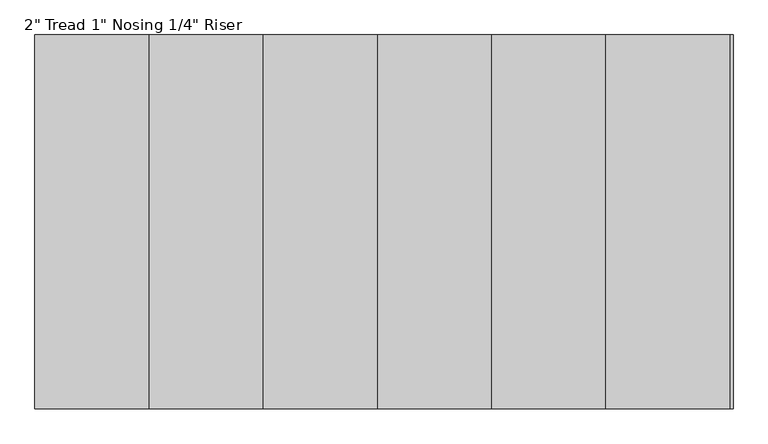
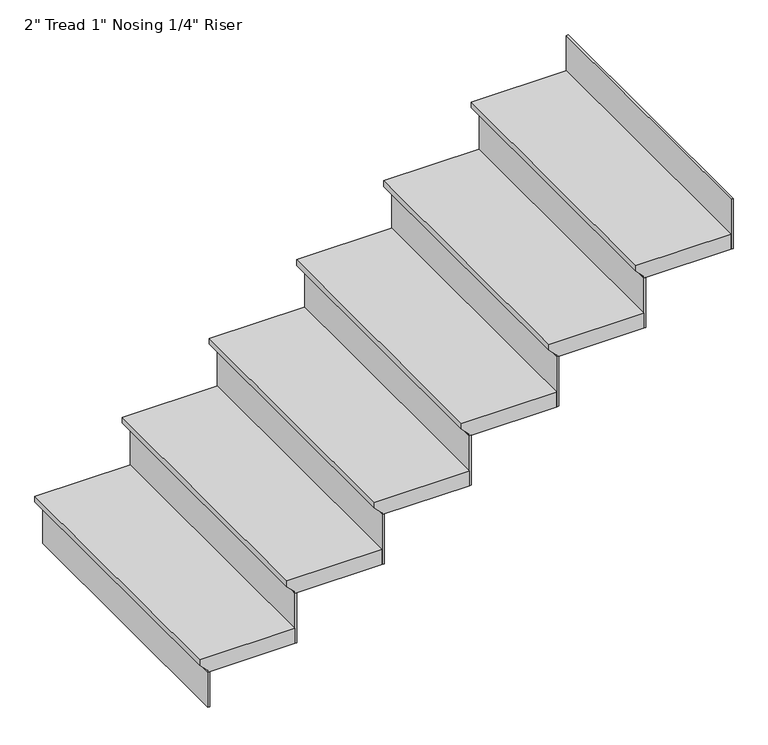
"""IFC4 building model written with IfcOpenShell, lengths in millimetres: stair flight geometry."""

from ifc_helpers import new_model, si_unit, frame, origin, place, context, project, spatial, polyline, outline, extrude, source, transform, mapped, element, save


def stair_flight_60bc6d16(model_context):
    return source(origin(), model_context, "Body", "SweptSolid", [
        extrude(outline(polyline([(3217.3333333, 1323.7430349), (3217.3333333, 1018.9430349), (3198.2833333, 1018.9430349), (3172.8833333, 1044.3430349), (3166.5333333, 1044.3430349), (3166.5333333, 1323.7430349), (3217.3333333, 1323.7430349)])), frame((0.0, 4166.2555142, 0.0), z_axis=(0.0, 1.0, 0.0), x_axis=(0.0, 0.0, 1.0)), (0.0, 0.0, 1.0), 914.4),
        extrude(outline(polyline([(1050.6930349, 4166.2555142), (1044.3430349, 4166.2555142), (1044.3430349, 5080.6555142), (1050.6930349, 5080.6555142), (1050.6930349, 4166.2555142)])), frame((0.0, 0.0, 3048.0), z_axis=(0.0, 0.0, 1.0), x_axis=(1.0, 0.0, 0.0)), (0.0, 0.0, 1.0), 118.5333333),
        extrude(outline(polyline([(1330.0930349, 4166.2555142), (1323.7430349, 4166.2555142), (1323.7430349, 5080.6555142), (1330.0930349, 5080.6555142), (1330.0930349, 4166.2555142)])), frame((0.0, 0.0, 3166.5333333), z_axis=(0.0, 0.0, 1.0), x_axis=(1.0, 0.0, 0.0)), (0.0, 0.0, 1.0), 169.3333333),
        extrude(outline(polyline([(3386.6666667, 1603.1430349), (3386.6666667, 1298.3430349), (3367.6166667, 1298.3430349), (3342.2166667, 1323.7430349), (3335.8666667, 1323.7430349), (3335.8666667, 1603.1430349), (3386.6666667, 1603.1430349)])), frame((0.0, 4166.2555142, 0.0), z_axis=(0.0, 1.0, 0.0), x_axis=(0.0, 0.0, 1.0)), (0.0, 0.0, 1.0), 914.4),
        extrude(outline(polyline([(1609.4930349, 4166.2555142), (1603.1430349, 4166.2555142), (1603.1430349, 5080.6555142), (1609.4930349, 5080.6555142), (1609.4930349, 4166.2555142)])), frame((0.0, 0.0, 3335.8666667), z_axis=(0.0, 0.0, 1.0), x_axis=(1.0, 0.0, 0.0)), (0.0, 0.0, 1.0), 169.3333333),
        extrude(outline(polyline([(3556.0, 1882.5430349), (3556.0, 1577.7430349), (3536.95, 1577.7430349), (3511.55, 1603.1430349), (3505.2, 1603.1430349), (3505.2, 1882.5430349), (3556.0, 1882.5430349)])), frame((0.0, 4166.2555142, 0.0), z_axis=(0.0, 1.0, 0.0), x_axis=(0.0, 0.0, 1.0)), (0.0, 0.0, 1.0), 914.4),
        extrude(outline(polyline([(1888.8930349, 4166.2555142), (1882.5430349, 4166.2555142), (1882.5430349, 5080.6555142), (1888.8930349, 5080.6555142), (1888.8930349, 4166.2555142)])), frame((0.0, 0.0, 3505.2), z_axis=(0.0, 0.0, 1.0), x_axis=(1.0, 0.0, 0.0)), (0.0, 0.0, 1.0), 169.3333333),
        extrude(outline(polyline([(3725.3333333, 2161.9430349), (3725.3333333, 1857.1430349), (3706.2833333, 1857.1430349), (3680.8833333, 1882.5430349), (3674.5333333, 1882.5430349), (3674.5333333, 2161.9430349), (3725.3333333, 2161.9430349)])), frame((0.0, 4166.2555142, 0.0), z_axis=(0.0, 1.0, 0.0), x_axis=(0.0, 0.0, 1.0)), (0.0, 0.0, 1.0), 914.4),
        extrude(outline(polyline([(2168.2930349, 4166.2555142), (2161.9430349, 4166.2555142), (2161.9430349, 5080.6555142), (2168.2930349, 5080.6555142), (2168.2930349, 4166.2555142)])), frame((0.0, 0.0, 3674.5333333), z_axis=(0.0, 0.0, 1.0), x_axis=(1.0, 0.0, 0.0)), (0.0, 0.0, 1.0), 169.3333333),
        extrude(outline(polyline([(3894.6666667, 2441.3430349), (3894.6666667, 2136.5430349), (3875.6166667, 2136.5430349), (3850.2166667, 2161.9430349), (3843.8666667, 2161.9430349), (3843.8666667, 2441.3430349), (3894.6666667, 2441.3430349)])), frame((0.0, 4166.2555142, 0.0), z_axis=(0.0, 1.0, 0.0), x_axis=(0.0, 0.0, 1.0)), (0.0, 0.0, 1.0), 914.4),
        extrude(outline(polyline([(2447.6930349, 4166.2555142), (2441.3430349, 4166.2555142), (2441.3430349, 5080.6555142), (2447.6930349, 5080.6555142), (2447.6930349, 4166.2555142)])), frame((0.0, 0.0, 3843.8666667), z_axis=(0.0, 0.0, 1.0), x_axis=(1.0, 0.0, 0.0)), (0.0, 0.0, 1.0), 169.3333333),
        extrude(outline(polyline([(4064.0, 2720.7430349), (4064.0, 2415.9430349), (4044.95, 2415.9430349), (4019.55, 2441.3430349), (4013.2, 2441.3430349), (4013.2, 2720.7430349), (4064.0, 2720.7430349)])), frame((0.0, 4166.2555142, 0.0), z_axis=(0.0, 1.0, 0.0), x_axis=(0.0, 0.0, 1.0)), (0.0, 0.0, 1.0), 914.4),
        extrude(outline(polyline([(2727.0930349, 4166.2555142), (2720.7430349, 4166.2555142), (2720.7430349, 5080.6555142), (2727.0930349, 5080.6555142), (2727.0930349, 4166.2555142)])), frame((0.0, 0.0, 4013.2), z_axis=(0.0, 0.0, 1.0), x_axis=(1.0, 0.0, 0.0)), (0.0, 0.0, 1.0), 169.3333333),
    ])


if __name__ == "__main__":
    model = new_model("IFC4")
    model_context = context("Model", 3, world=origin())
    ifc_project = project(units=[si_unit("LENGTHUNIT", "METRE", prefix="MILLI")], contexts=[model_context])
    site = spatial("IfcSite", under=ifc_project)
    building = spatial("IfcBuilding", under=site)
    placement = place(None, origin())
    stair_flight_shape = stair_flight_60bc6d16(model_context)
    element("IfcStairFlight", 1, ObjectType="2\" Tread 1\" Nosing 1/4\" Riser", at=placement, inside=building, context=model_context, shape_type="MappedRepresentation", body=[
        mapped(stair_flight_shape, transform((0.0, 0.0, 0.0), x_axis=(1.0, 0.0, 0.0), y_axis=(0.0, 1.0, 0.0), z_axis=(0.0, 0.0, 1.0))),
    ])
    save(model, "model.ifc")
